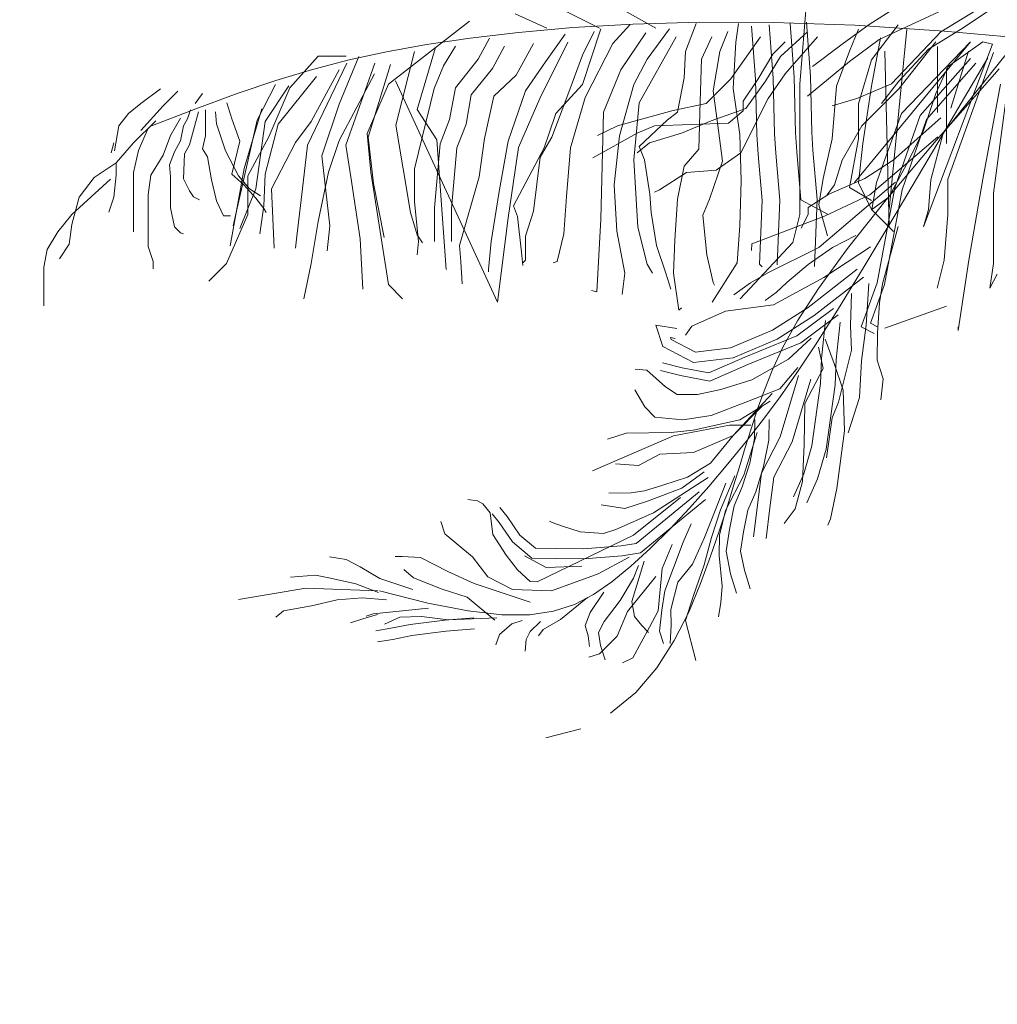
# Model space of a CAD drawing. Units: millimetres. Extents: x 595116 to 630915, y 909473 to 920225.
# Tile 67 of 134: x 629618.94 to 629629.07, y 919266.51 to 919276.71. Entities that reach past the tile are written whole.
import ezdxf

# ---------------------------------------------------------------- set-up
doc = ezdxf.new("R2010")
doc.units = ezdxf.units.MM
doc.layers.add('Dimension', color=3, linetype='Continuous', lineweight=18)
doc.layers.add('L-PLNT', color=85, linetype='Continuous', lineweight=13)
doc.styles.get("Standard").update_dxf_attribs({"font": 'arial.ttf'})
doc.dimstyles.new('ISO-25', dxfattribs={"dimtxt": 9, "dimasz": 6, "dimexe": 1.25, "dimexo": 0.625, "dimtad": 1, "dimlunit": 4, "dimtxsty": 'Standard', "dimcen": 2.5, "dimadec": 0, "dimazin": 0, "dimtfac": 1, "dimtmove": 0, "dimatfit": 3, "dimfxl": 1, "dimarcsym": 0})

# ---------------------------------------------------------------- blocks, each defined once
blk = doc.blocks.new('A$C4FB75ABC')
for p, q in [((2.1065, 2.3741), (2.087, 2.1315)), ((2.2781, 2.2963), (2.353, 2.344)), ((2.5983, 2.3508), (2.4757, 2.2759)), ((1.3881, 2.2867), (1.3008, 2.3255)), ((1.5337, 2.2867), (1.4367, 2.3352)), ((1.6891, 2.2867), (1.6017, 2.3352)), ((2.3054, 2.2555), (2.4825, 2.3372)), ((2.6119, 2.3372), (2.5302, 2.2827)), ((1.1746, 2.3061), (0.9513, 2.1315)), ((1.4598, 2.2878), (1.3106, 2.2744)), ((1.6258, 2.2976), (1.4598, 2.2878)), ((1.5376, 2.2844), (1.4866, 2.1313)), ((1.6179, 2.2954), (1.5705, 2.2443)), ((1.8099, 2.3026), (1.6258, 2.2976)), ((1.7274, 2.2844), (1.6654, 2.2006)), ((1.8004, 2.299), (1.7712, 2.2224)), ((2.0136, 2.3019), (1.8099, 2.3026)), ((1.9171, 2.299), (1.9098, 2.248)), ((1.9536, 2.2917), (1.9646, 2.1459)), ((2.0023, 2.2954), (2.0134, 2.1483)), ((2.2382, 2.2942), (2.0136, 2.3019)), ((2.0597, 2.2997), (2.0708, 2.1511)), ((2.1047, 2.3031), (2.1159, 2.1533)), ((2.2032, 2.2419), (2.2781, 2.2963)), ((2.2482, 2.2839), (2.2239, 2.2232)), ((2.4852, 2.2785), (2.2382, 2.2942)), ((2.3575, 2.296), (2.2846, 2.199)), ((2.3818, 2.2839), (2.3332, 1.7863)), ((1.1767, 2.2586), (1.0564, 2.241)), ((1.3106, 2.2744), (1.1767, 2.2586)), ((1.23, 2.2589), (1.1992, 2.2008)), ((1.4391, 2.2699), (1.3844, 2.1933)), ((1.5194, 2.2771), (1.4866, 2.2115)), ((1.6617, 2.2735), (1.5924, 2.1714)), ((1.7456, 2.2626), (1.6435, 2.0802)), ((1.8442, 2.2626), (1.815, 2.2006)), ((1.8879, 2.2771), (1.8661, 2.2224)), ((1.9783, 2.2623), (1.8966, 2.1465)), ((2.1078, 2.2759), (2.0328, 2.2078)), ((2.135, 2.2623), (2.0465, 2.1602)), ((2.3089, 2.2596), (2.2846, 2.1261)), ((2.4757, 2.2759), (2.3394, 2.1329)), ((2.5302, 2.2827), (2.4416, 2.2282)), ((2.6937, 2.2623), (2.4825, 1.9967)), ((2.7559, 2.2536), (2.4852, 2.2785)), ((1.0564, 2.241), (0.9464, 2.2213)), ((1.0815, 2.2334), (1.0304, 2.062)), ((1.1363, 2.237), (1.1034, 2.1823)), ((1.2713, 2.237), (1.2384, 2.175)), ((1.3515, 2.2443), (1.3041, 2.1568)), ((1.4464, 2.2479), (1.3687, 2.0927)), ((1.5705, 2.2443), (1.4939, 2.0948)), ((1.9098, 2.248), (1.9025, 2.1203)), ((2.0124, 2.2146), (2.0465, 2.2487)), ((2.1214, 2.1806), (2.2032, 2.2419)), ((2.2236, 2.1942), (2.3054, 2.2555)), ((2.5574, 2.2487), (2.2372, 1.8605)), ((2.462, 2.2487), (2.3599, 2.1193)), ((2.3667, 2.0512), (2.5574, 2.2487)), ((2.428, 1.738), (2.6187, 2.2419)), ((2.4668, 2.2354), (2.4668, 2.0533)), ((2.5915, 2.2487), (2.4961, 2.1806)), ((2.6187, 2.2419), (2.5915, 2.2487)), ((0.7572, 2.2091), (0.6795, 2.1218)), ((0.8348, 2.2091), (0.7572, 2.2091)), ((0.8699, 2.2079), (0.8151, 2.0766)), ((0.9464, 2.2213), (0.8429, 2.1986)), ((1.0231, 2.2224), (0.972, 2.0182)), ((1.4866, 2.2115), (1.4464, 2.1021)), ((1.7712, 2.2224), (1.7675, 2.1495)), ((1.8661, 2.2224), (1.8478, 2.113)), ((1.9715, 2.1465), (2.0124, 2.2146)), ((2.0328, 2.2078), (1.992, 2.1397)), ((2.2239, 2.2232), (2.1875, 2.1261)), ((2.3211, 2.2232), (2.3332, 1.7378)), ((2.4416, 2.2282), (2.3599, 2.1397)), ((2.5572, 2.203), (2.4187, 2.0449)), ((2.6056, 2.2048), (2.4676, 1.9701)), ((2.6209, 2.2188), (2.4948, 1.8695)), ((2.5518, 2.2232), (2.5032, 2.0655)), ((0.837, 2.1896), (0.7276, 1.9635)), ((0.8429, 2.1986), (0.7422, 2.1723)), ((0.9137, 2.1896), (0.8334, 1.9635)), ((0.9575, 2.186), (0.8954, 1.9854)), ((1.1034, 2.1823), (1.0779, 2.1203)), ((1.1992, 2.2008), (1.1362, 2.1221)), ((1.2384, 2.175), (1.18, 2.1021)), ((1.3844, 2.1933), (1.3297, 2.113)), ((1.6654, 2.2006), (1.6289, 2.1313)), ((1.815, 2.2006), (1.8113, 2.0838)), ((2.1078, 2.0989), (2.2236, 2.1942)), ((2.2846, 2.199), (2.2482, 2.0776)), ((2.5724, 2.1897), (2.4365, 2.0345)), ((2.4961, 2.1806), (2.462, 2.1057)), ((2.6368, 2.1742), (2.4628, 1.9766)), ((2.4911, 2.1747), (2.4911, 1.9684)), ((0.7422, 2.1723), (0.6405, 2.1416)), ((0.7531, 2.1531), (0.6473, 2.0218)), ((0.8151, 2.1714), (0.7385, 2.0291)), ((0.9125, 2.1606), (0.8154, 1.9763)), ((1.3041, 2.1568), (1.2421, 2.0984)), ((1.5924, 2.1714), (1.5449, 2.0547)), ((1.7675, 2.1495), (1.7493, 2.0547)), ((2.0465, 2.1602), (1.9988, 2.0921)), ((2.0134, 2.1483), (2.017, 1.9949)), ((2.0708, 2.1511), (2.0745, 1.9975)), ((2.1159, 2.1533), (2.1196, 1.9995)), ((0.6405, 2.1416), (0.5342, 2.1057)), ((0.64, 2.1313), (0.5889, 2.0328)), ((0.6765, 2.1276), (0.6108, 2.0291)), ((0.6795, 2.1218), (0.6213, 1.986)), ((0.9513, 2.1315), (0.8931, 1.9957)), ((1.2522, 1.53), (0.9707, 2.1412)), ((1.0779, 2.1203), (1.0231, 1.8978)), ((1.1362, 2.1221), (1.1203, 2.0346)), ((1.4866, 2.1313), (1.4136, 2.051)), ((1.6289, 2.1313), (1.5887, 1.989)), ((1.8966, 2.1465), (1.8285, 2.0784)), ((1.9025, 2.1203), (1.9208, 1.9927)), ((1.9306, 2.0852), (1.9715, 2.1465)), ((1.992, 2.1397), (1.9375, 2.0648)), ((1.9646, 2.1459), (1.9682, 1.9927)), ((2.087, 2.1315), (2.087, 1.7725)), ((2.1875, 2.1261), (2.1754, 1.9805)), ((2.3394, 2.1329), (2.244, 2.0921)), ((2.2846, 2.1261), (2.2604, 1.9684)), ((2.3599, 2.1397), (2.3122, 2.0784)), ((2.6404, 2.1315), (2.5918, 1.8695)), ((2.6598, 2.1218), (2.6209, 1.8307)), ((0.2683, 2.0784), (0.3228, 2.1193)), ((0.3296, 2.0716), (0.3705, 2.1125)), ((0.4182, 2.0784), (0.4386, 2.1057)), ((0.5342, 2.1057), (0.4195, 2.0639)), ((1.18, 2.1021), (1.1654, 2.0218)), ((1.2421, 2.0984), (1.2165, 1.9817)), ((1.3297, 2.113), (1.2822, 1.9744)), ((1.3687, 2.0927), (1.3105, 1.9569)), ((1.4464, 2.1021), (1.4026, 1.9854)), ((1.4939, 2.0948), (1.4537, 1.9562)), ((1.8478, 2.113), (1.8624, 2.0036)), ((2.3599, 2.1193), (2.2577, 2.0172)), ((2.462, 2.1057), (2.428, 2.0035)), ((0.2342, 2.0512), (0.2683, 2.0784)), ((0.2683, 2.0035), (0.3296, 2.0716)), ((0.505, 2.0802), (0.5196, 2.0364)), ((0.8151, 2.0766), (0.7677, 1.9343)), ((1.6435, 2.0802), (1.6289, 1.9234)), ((1.8285, 2.0784), (1.7331, 2.058)), ((1.8113, 2.0838), (1.8077, 1.9526)), ((1.9988, 2.0921), (1.9238, 1.9422)), ((1.9306, 2.058), (1.9306, 2.0852)), ((2.244, 2.0921), (2.1759, 2.0716)), ((2.2482, 2.0776), (2.2482, 1.9805)), ((0.207, 2.0172), (0.2342, 2.0512)), ((0.4195, 2.0639), (0.2927, 2.0154)), ((0.4049, 2.0609), (0.3966, 2.0361)), ((0.427, 2.0554), (0.4021, 1.9643)), ((0.4463, 2.0609), (0.4463, 1.9892)), ((0.4739, 2.0554), (0.4767, 2.0223)), ((0.6018, 2.0636), (0.5533, 1.8986)), ((1.0304, 2.062), (1.0852, 1.9781)), ((1.4136, 2.051), (1.3953, 1.9963)), ((1.5449, 2.0547), (1.5376, 1.7593)), ((1.7331, 2.058), (1.5832, 2.0172)), ((1.7493, 2.0547), (1.7201, 2.0328)), ((1.9375, 2.0648), (1.8421, 2.0308)), ((1.8898, 2.024), (1.9306, 2.058)), ((2.2985, 1.8605), (2.3667, 2.0512)), ((2.4756, 2.0387), (2.3438, 1.9217)), ((2.4187, 2.0449), (2.3489, 1.8456)), ((0.195, 1.9478), (0.207, 2.0172)), ((0.3092, 2.0308), (0.2479, 1.9695)), ((0.3773, 2.0376), (0.3501, 1.9899)), ((0.3855, 2.0168), (0.3773, 1.9754)), ((0.3966, 2.0361), (0.3855, 2.0168)), ((0.4767, 2.0223), (0.5015, 1.9478)), ((0.5196, 2.0364), (0.5415, 1.9744)), ((0.5889, 2.0328), (0.5232, 1.741)), ((0.6108, 2.0291), (0.5853, 1.8431)), ((0.6473, 2.0218), (0.6108, 1.8833)), ((0.7385, 2.0291), (0.6947, 1.9708)), ((0.972, 2.0182), (1.0122, 1.7775)), ((1.1203, 2.0346), (1.0939, 1.9669)), ((1.1654, 2.0218), (1.1399, 1.9562)), ((1.5832, 2.0172), (1.5287, 1.9899)), ((1.6377, 1.9967), (1.6854, 2.0172)), ((1.7201, 2.0328), (1.6435, 1.9598)), ((1.6854, 2.0172), (1.8898, 2.024)), ((1.8421, 2.0308), (1.7603, 1.9967)), ((2.2577, 2.0172), (2.2032, 1.9218)), ((2.4365, 2.0345), (2.3686, 1.8404)), ((0.2887, 2.0103), (0.2615, 1.9491)), ((0.3501, 1.9899), (0.3296, 1.9354)), ((0.4463, 1.9892), (0.438, 1.9533)), ((0.6213, 1.986), (0.563, 1.8792)), ((0.8931, 1.9957), (0.9028, 1.8889)), ((0.8954, 1.9854), (0.91, 1.8577)), ((1.4026, 1.9854), (1.3698, 1.9307)), ((1.3953, 1.9963), (1.3807, 1.9562)), ((1.5151, 1.9286), (1.6377, 1.9967)), ((1.5887, 1.989), (1.5741, 1.8541)), ((1.7603, 1.9967), (1.6718, 1.9695)), ((1.8624, 2.0036), (1.8734, 1.9197)), ((1.9208, 1.9927), (1.9244, 1.865)), ((1.9682, 1.9927), (1.9719, 1.938)), ((2.017, 1.9949), (2.0206, 1.9417)), ((2.0745, 1.9975), (2.0779, 1.946)), ((2.1196, 1.9995), (2.1229, 1.9495)), ((2.4673, 1.986), (2.2802, 1.8264)), ((2.428, 2.0035), (2.3871, 1.9218)), ((2.4825, 1.9967), (2.4484, 1.8673)), ((0.1865, 1.9422), (0.1934, 1.9695)), ((0.2479, 1.9695), (0.2002, 1.915)), ((0.3773, 1.9754), (0.3607, 1.945)), ((0.4021, 1.9643), (0.3883, 1.9395)), ((0.5415, 1.9744), (0.5196, 1.8833)), ((0.6947, 1.9708), (0.629, 1.8431)), ((0.7276, 1.9635), (0.713, 1.8358)), ((0.8154, 1.9763), (0.7863, 1.8889)), ((0.8334, 1.9635), (0.848, 1.876)), ((1.0939, 1.9669), (1.0786, 1.7905)), ((1.0852, 1.9781), (1.1107, 1.6207)), ((1.2165, 1.9817), (1.2019, 1.876)), ((1.2822, 1.9744), (1.2567, 1.8358)), ((1.3105, 1.9569), (1.2814, 1.7628)), ((1.6718, 1.9695), (1.6377, 1.9422)), ((1.6435, 1.9598), (1.6581, 1.9234)), ((2.1754, 1.9805), (2.1511, 1.8713)), ((2.2482, 1.9805), (2.2239, 1.847)), ((2.2604, 1.9684), (2.2482, 1.8591)), ((2.4628, 1.9766), (2.3249, 1.8127)), ((2.4676, 1.9701), (2.3552, 1.7802)), ((0.2615, 1.9491), (0.2479, 1.8878)), ((0.3296, 1.9354), (0.2956, 1.881)), ((0.3607, 1.945), (0.3469, 1.9091)), ((0.3883, 1.9395), (0.3855, 1.8705)), ((0.438, 1.9533), (0.4518, 1.9312)), ((0.4518, 1.9312), (0.4629, 1.8677)), ((0.5015, 1.9478), (0.5374, 1.8788)), ((0.7677, 1.9343), (0.7896, 1.741)), ((1.1399, 1.9562), (1.1253, 1.7884)), ((1.3807, 1.9562), (1.2968, 1.7957)), ((1.3698, 1.9307), (1.3515, 1.7811)), ((1.4537, 1.9562), (1.4428, 1.8213)), ((1.8077, 1.9526), (1.7675, 1.9051)), ((1.9238, 1.9422), (1.8557, 1.8946)), ((1.9719, 1.938), (1.9828, 1.8103)), ((2.0206, 1.9417), (2.0317, 1.8114)), ((2.0779, 1.946), (2.0893, 1.8127)), ((2.1229, 1.9495), (2.1345, 1.8136)), ((0.2002, 1.915), (0.1389, 1.8742)), ((0.2002, 1.915), (0.2002, 1.881)), ((0.3469, 1.9091), (0.3497, 1.876)), ((1.6289, 1.9234), (1.6398, 1.7374)), ((1.6581, 1.9234), (1.6727, 1.8285)), ((1.7675, 1.9051), (1.7493, 1.814)), ((1.8734, 1.9197), (1.8369, 1.814)), ((2.2032, 1.9218), (2.1827, 1.8537)), ((2.3438, 1.9217), (2.2657, 1.8718)), ((2.3871, 1.9218), (2.3326, 1.8197)), ((0.2002, 1.881), (0.1934, 1.8197)), ((0.2479, 1.8878), (0.2479, 1.8061)), ((0.2956, 1.881), (0.2887, 1.8265)), ((0.3497, 1.876), (0.3497, 1.8512)), ((0.5196, 1.8833), (0.5524, 1.8541)), ((0.5533, 1.8986), (0.5339, 1.7919)), ((0.5374, 1.8788), (0.5678, 1.8429)), ((0.563, 1.8792), (0.563, 1.7725)), ((0.6108, 1.8833), (0.6072, 1.7957)), ((0.7863, 1.8889), (0.7572, 1.7531)), ((0.848, 1.876), (0.8735, 1.7045)), ((0.9028, 1.8889), (0.9513, 1.5785)), ((1.0231, 1.8978), (1.0231, 1.8067)), ((1.2019, 1.876), (1.1472, 1.6863)), ((1.7739, 1.8878), (1.699, 1.8401)), ((1.8557, 1.8946), (1.7739, 1.8878)), ((0.1844, 1.8695), (0.0777, 1.7725)), ((0.1389, 1.8742), (0.098, 1.8197)), ((0.3497, 1.8512), (0.3497, 1.7904)), ((0.3855, 1.8705), (0.4021, 1.8374)), ((0.4629, 1.8677), (0.4767, 1.8098)), ((0.5524, 1.8541), (0.5853, 1.8176)), ((0.91, 1.8577), (0.9392, 1.7082)), ((1.5741, 1.8541), (1.5814, 1.7264)), ((1.9244, 1.865), (1.9208, 1.741)), ((2.3505, 1.8613), (2.1386, 1.6813)), ((2.1511, 1.8713), (2.1389, 1.7985)), ((2.1827, 1.8537), (2.1623, 1.8265)), ((2.2657, 1.8718), (2.167, 1.8279)), ((2.2482, 1.8591), (2.2846, 1.7863)), ((2.2849, 1.7856), (2.2985, 1.8605)), ((2.4484, 1.8673), (2.4416, 1.7856)), ((2.4948, 1.8695), (2.4948, 1.7725)), ((2.5918, 1.8695), (2.553, 1.6464)), ((0.2887, 1.8265), (0.2887, 1.7516)), ((0.4021, 1.8374), (0.4132, 1.8208)), ((0.5853, 1.8431), (0.5415, 1.7337)), ((0.5678, 1.8429), (0.5982, 1.8236)), ((0.629, 1.8431), (0.6363, 1.679)), ((0.713, 1.8358), (0.6984, 1.7118)), ((1.2567, 1.8358), (1.2348, 1.6973)), ((1.4428, 1.8213), (1.4355, 1.7191)), ((1.6727, 1.8285), (1.6763, 1.7775)), ((1.699, 1.8401), (1.6854, 1.8333)), ((2.167, 1.8279), (2.1099, 1.791)), ((2.2802, 1.8264), (2.1549, 1.7678)), ((2.2239, 1.847), (2.2846, 1.8106)), ((2.3489, 1.8456), (2.3004, 1.5838)), ((2.3686, 1.8404), (2.32, 1.5785)), ((2.6209, 1.8307), (2.6209, 1.6367)), ((0.098, 1.8197), (0.0775, 1.7448)), ((0.1934, 1.8197), (0.1797, 1.7788)), ((0.2479, 1.8061), (0.2479, 1.7448)), ((0.4132, 1.8208), (0.4297, 1.8125)), ((0.4767, 1.8098), (0.496, 1.7684)), ((0.5853, 1.8176), (0.6072, 1.7884)), ((0.6072, 1.7957), (0.5962, 1.7191)), ((1.0231, 1.8067), (1.0341, 1.6973)), ((1.2968, 1.7957), (1.3078, 1.7665)), ((1.7493, 1.814), (1.742, 1.7009)), ((1.8369, 1.814), (1.8186, 1.7702)), ((1.9828, 1.8103), (1.9755, 1.6352)), ((2.0317, 1.8114), (2.0243, 1.6332)), ((2.0893, 1.8127), (2.1647, 1.7725)), ((2.1345, 1.8136), (2.1268, 1.6289)), ((2.1389, 1.7985), (2.1632, 1.7135)), ((2.3249, 1.8127), (2.2184, 1.678)), ((2.3326, 1.8197), (2.2849, 1.7856)), ((0.0777, 1.7725), (0.0388, 1.724)), ((0.3497, 1.7904), (0.3607, 1.738)), ((0.496, 1.7684), (0.5153, 1.7684)), ((0.563, 1.7725), (0.5048, 1.6367)), ((0.5339, 1.7919), (0.5145, 1.6852)), ((0.6072, 1.7884), (0.6144, 1.7775)), ((1.0122, 1.7775), (1.0304, 1.7155)), ((1.0786, 1.7905), (1.0786, 1.6973)), ((1.1253, 1.7884), (1.1253, 1.7665)), ((1.1253, 1.7665), (1.1253, 1.7301)), ((1.3078, 1.7665), (1.3187, 1.6681)), ((1.3515, 1.7811), (1.3297, 1.7118)), ((1.6763, 1.7775), (1.6909, 1.6863)), ((1.8186, 1.7702), (1.8296, 1.6608)), ((2.1549, 1.7678), (1.9538, 1.6913)), ((2.087, 1.7725), (2.0676, 1.6949)), ((2.1096, 1.7722), (2.0903, 1.7347)), ((2.1099, 1.791), (2.1096, 1.7722)), ((2.3552, 1.7802), (2.2641, 1.6283)), ((2.2846, 1.7863), (2.3453, 1.7256)), ((2.4416, 1.7856), (2.428, 1.738)), ((2.4948, 1.7725), (2.485, 1.6464)), ((0.0775, 1.7448), (0.0707, 1.6903)), ((0.2479, 1.7448), (0.2479, 1.7243)), ((0.2887, 1.7516), (0.2887, 1.6835)), ((0.7572, 1.7531), (0.7377, 1.6367)), ((0.7896, 1.741), (0.7823, 1.6717)), ((1.2814, 1.7628), (1.2522, 1.53)), ((1.5376, 1.7593), (1.5267, 1.5587)), ((1.9208, 1.741), (1.9135, 1.6389)), ((0.0388, 1.724), (0.0097, 1.6755)), ((0.3607, 1.738), (0.3773, 1.7214)), ((0.3773, 1.7214), (0.3855, 1.7187)), ((1.0304, 1.7155), (1.045, 1.6936)), ((1.1253, 1.7301), (1.1253, 1.6973)), ((1.4355, 1.7191), (1.4172, 1.6425)), ((1.5814, 1.7264), (1.6033, 1.6097)), ((1.6398, 1.7374), (1.6654, 1.6352)), ((2.2409, 1.7138), (2.1763, 1.6807)), ((2.3582, 1.7386), (2.3145, 1.5808)), ((0.0707, 1.6903), (0.0435, 1.6494)), ((0.6984, 1.7118), (0.6947, 1.679)), ((0.8735, 1.7045), (0.8808, 1.566)), ((1.0341, 1.6973), (1.0304, 1.6608)), ((1.1472, 1.6863), (1.1509, 1.6425)), ((1.2348, 1.6973), (1.2275, 1.6207)), ((1.3297, 1.7118), (1.3297, 1.6462)), ((1.6909, 1.6863), (1.7164, 1.6097)), ((1.742, 1.7009), (1.7383, 1.6097)), ((2.0676, 1.6949), (1.922, 1.5397)), ((1.9538, 1.6913), (1.9536, 1.6725)), ((0.0097, 1.6755), (0, 1.627)), ((0.2887, 1.6835), (0.3024, 1.6426)), ((1.3187, 1.6681), (1.3224, 1.6316)), ((1.8296, 1.6608), (1.8478, 1.5842)), ((2.1386, 1.6813), (1.998, 1.6115)), ((2.1763, 1.6807), (2.1096, 1.6345)), ((2.2184, 1.678), (2.1385, 1.568)), ((2.2819, 1.6831), (2.1525, 1.5981)), ((0.3024, 1.6426), (0.3024, 1.6222)), ((0.5048, 1.6367), (0.4562, 1.5882)), ((0.7377, 1.6367), (0.7183, 1.5397)), ((1.1509, 1.6425), (1.1545, 1.5805)), ((1.3297, 1.6462), (1.3224, 1.6389)), ((1.4172, 1.6425), (1.4063, 1.6389)), ((1.6654, 1.6352), (1.68, 1.6097)), ((1.9135, 1.6389), (1.8444, 1.53)), ((1.9755, 1.6352), (1.9828, 1.628)), ((2.1096, 1.6345), (2.0504, 1.5844)), ((2.485, 1.6464), (2.4656, 1.5688)), ((2.553, 1.6464), (2.5239, 1.4523)), ((2.6209, 1.6367), (2.6112, 1.5688)), ((0, 1.627), (0, 1.5494)), ((1.2275, 1.6207), (1.2275, 1.6134)), ((1.6033, 1.6097), (1.596, 1.5514)), ((1.7164, 1.6097), (1.731, 1.566)), ((1.7383, 1.6097), (1.7529, 1.5076)), ((1.998, 1.6115), (1.9504, 1.5839)), ((2.2452, 1.6213), (2.1098, 1.5157)), ((2.2641, 1.6283), (2.1904, 1.5079)), ((2.6112, 1.5688), (2.6307, 1.6076)), ((0.9513, 1.5785), (0.9901, 1.5397)), ((1.8478, 1.5842), (1.8515, 1.5769)), ((1.9504, 1.5839), (1.9047, 1.5506)), ((2.1525, 1.5981), (2.0137, 1.5227)), ((2.0504, 1.5844), (2.0217, 1.5565)), ((2.2623, 1.5995), (2.1258, 1.493)), ((2.3004, 1.5838), (2.256, 1.4617)), ((2.2767, 1.5813), (2.2695, 1.4664)), ((2.32, 1.5785), (2.2812, 1.4717)), ((2.3145, 1.5808), (2.3062, 1.5281)), ((0, 1.5494), (0, 1.5203)), ((1.5267, 1.5587), (1.5121, 1.5623)), ((2.0217, 1.5565), (1.9912, 1.5343)), ((2.1385, 1.568), (2.0803, 1.4783)), ((2.2292, 1.5537), (2.2261, 1.4651)), ((2.0137, 1.5227), (1.8814, 1.5056)), ((2.3062, 1.5281), (2.3013, 1.4452)), ((1.7529, 1.5076), (1.7602, 1.5149)), ((1.8814, 1.5056), (1.7884, 1.4636)), ((2.1098, 1.5157), (2.0109, 1.453)), ((2.1796, 1.5129), (2.0785, 1.437)), ((2.1927, 1.4954), (2.0894, 1.4177)), ((2.1904, 1.5079), (2.1298, 1.4122)), ((2.4911, 1.5193), (2.3211, 1.4586)), ((2.1258, 1.493), (2.0238, 1.4284)), ((2.0803, 1.4783), (2.039, 1.4043)), ((2.1578, 1.4791), (2.1468, 1.3743)), ((2.1979, 1.4749), (2.187, 1.3714)), ((2.2812, 1.4717), (2.3006, 1.462)), ((1.7084, 1.4073), (1.6895, 1.4666)), ((1.6895, 1.4666), (1.747, 1.4576)), ((1.7884, 1.4636), (1.7711, 1.4393)), ((2.0109, 1.453), (1.8951, 1.4036)), ((2.2261, 1.4651), (2.2289, 1.3972)), ((2.256, 1.4617), (2.2916, 1.4439)), ((2.2695, 1.4664), (2.2568, 1.3685)), ((2.3013, 1.4452), (2.3002, 1.3698)), ((2.5239, 1.4523), (2.5239, 1.462)), ((1.7313, 1.4266), (1.7295, 1.4323)), ((1.7295, 1.4323), (1.7427, 1.4302)), ((1.7987, 1.3918), (1.7313, 1.4266)), ((2.0238, 1.4284), (1.9024, 1.3766)), ((2.0785, 1.437), (1.9344, 1.3786)), ((2.0894, 1.4177), (1.9429, 1.3584)), ((2.1181, 1.4308), (2.055, 1.3732)), ((2.1569, 1.4277), (2.1816, 1.3609)), ((1.7936, 1.3632), (1.7084, 1.4073)), ((1.8951, 1.4036), (1.7987, 1.3918)), ((2.039, 1.4043), (2.0098, 1.3416)), ((2.1298, 1.4122), (2.0784, 1.3347)), ((2.1385, 1.406), (2.1509, 1.3473)), ((2.2289, 1.3972), (2.1929, 1.2544)), ((1.7623, 1.3489), (1.7078, 1.3628)), ((1.9024, 1.3766), (1.7936, 1.3632)), ((1.9344, 1.3786), (1.8357, 1.3347)), ((2.055, 1.3732), (1.9542, 1.3161)), ((2.1468, 1.3743), (2.1439, 1.3053)), ((2.1816, 1.3609), (2.2062, 1.287)), ((2.187, 1.3714), (2.1842, 1.3016)), ((2.2568, 1.3685), (2.2516, 1.2668)), ((2.3002, 1.3698), (2.3165, 1.3187)), ((1.6641, 1.3427), (1.6321, 1.345)), ((1.7163, 1.2967), (1.6641, 1.3427)), ((1.7575, 1.3275), (1.7024, 1.3416)), ((1.8357, 1.3347), (1.7623, 1.3489)), ((1.9429, 1.3584), (1.8383, 1.3119)), ((2.0098, 1.3416), (1.9878, 1.2857)), ((2.0811, 1.3502), (2.0312, 1.2905)), ((2.0784, 1.3347), (2.0319, 1.2687)), ((2.1509, 1.3473), (2.1005, 1.25)), ((1.8383, 1.3119), (1.7575, 1.3275)), ((1.9542, 1.3161), (1.869, 1.289)), ((2.0829, 1.3276), (2.0324, 1.158)), ((2.1165, 1.3176), (2.065, 1.1449)), ((2.1439, 1.3053), (2.1195, 1.1332)), ((2.3165, 1.3187), (2.31, 1.2603)), ((1.6589, 1.2409), (1.6313, 1.2885)), ((1.7481, 1.2755), (1.7163, 1.2967)), ((1.869, 1.289), (1.8046, 1.2748)), ((2.0103, 1.2776), (1.903, 1.1622)), ((2.0312, 1.2905), (1.9421, 1.2559)), ((1.9878, 1.2857), (1.9691, 1.2327)), ((2.1842, 1.3016), (2.1591, 1.1247)), ((2.2062, 1.287), (2.2097, 1.1745)), ((1.8046, 1.2748), (1.7481, 1.2755)), ((1.9421, 1.2559), (1.8416, 1.2177)), ((2.0043, 1.257), (1.9206, 1.2053)), ((2.0319, 1.2687), (1.9864, 1.2075)), ((2.1929, 1.2544), (2.1754, 1.2112)), ((2.2516, 1.2668), (2.22, 1.1691)), ((1.6868, 1.2123), (1.6589, 1.2409)), ((1.9834, 1.244), (1.903, 1.1622)), ((1.9691, 1.2327), (1.952, 1.1808)), ((2.1005, 1.25), (2.0989, 1.1369)), ((1.7641, 1.2056), (1.6868, 1.2123)), ((1.8416, 1.2177), (1.7641, 1.2056)), ((1.9206, 1.2053), (1.792, 1.1769)), ((1.9864, 1.2075), (1.9386, 1.1458)), ((1.9621, 1.2066), (1.9614, 1.1536)), ((2.0017, 1.2061), (2.001, 1.1495)), ((2.1754, 1.2112), (2.1606, 1.1002)), ((1.7315, 1.1702), (1.607, 1.1681)), ((1.792, 1.1769), (1.7315, 1.1702)), ((1.7376, 1.1613), (1.8929, 1.1904)), ((1.8929, 1.1904), (1.9511, 1.1904)), ((1.9692, 1.1707), (1.9317, 1.0524)), ((1.952, 1.1808), (1.9358, 1.129)), ((2.2097, 1.1745), (2.1886, 1.0162)), ((1.5143, 1.0642), (1.7376, 1.1613)), ((1.607, 1.1681), (1.5558, 1.1518)), ((1.903, 1.1622), (1.793, 1.1147)), ((1.903, 1.1622), (1.8397, 1.0857)), ((1.9386, 1.1458), (1.8882, 1.0835)), ((1.9614, 1.1536), (1.9482, 1.0859)), ((2.0324, 1.158), (1.9806, 1.0581)), ((2.001, 1.1495), (1.9867, 1.0762)), ((2.065, 1.1449), (2.0146, 1.0475)), ((1.793, 1.1147), (1.7005, 1.1103)), ((1.9358, 1.129), (1.9198, 1.076)), ((2.0989, 1.1369), (2.0937, 1.0351)), ((2.1195, 1.1332), (2.0972, 1.056)), ((2.1591, 1.1247), (2.1353, 1.0421)), ((1.7005, 1.1103), (1.6416, 1.079)), ((1.6416, 1.079), (1.5775, 1.0837)), ((1.8224, 1.0615), (1.7614, 1.017)), ((1.8397, 1.0857), (1.7769, 1.047)), ((1.8882, 1.0835), (1.8359, 1.0215)), ((1.9198, 1.076), (1.903, 1.0206)), ((1.9482, 1.0859), (1.9278, 1.0204)), ((1.9867, 1.0762), (1.965, 1.0067)), ((1.8335, 1.0462), (1.6831, 0.9483)), ((1.7769, 1.047), (1.7087, 1.0253)), ((1.9071, 1.0509), (1.8681, 0.9571)), ((1.9317, 1.0524), (1.8813, 0.9551)), ((1.9806, 1.0581), (1.9586, 0.8825)), ((2.0146, 1.0475), (2.004, 0.9628)), ((2.0972, 1.056), (2.0692, 0.9929)), ((2.0937, 1.0351), (2.0738, 0.96)), ((2.1353, 1.0421), (2.1061, 0.9765)), ((1.6576, 1.009), (1.6216, 1.0039)), ((1.8084, 1.007), (1.6348, 0.8642)), ((1.7087, 1.0253), (1.6576, 1.009)), ((1.7614, 1.017), (1.6666, 0.9806)), ((1.8359, 1.0215), (1.7823, 0.9612)), ((1.8823, 1.0305), (1.8549, 0.9592)), ((1.903, 1.0206), (1.8847, 0.9618)), ((1.9278, 1.0204), (1.9055, 0.9679)), ((1.965, 1.0067), (1.9435, 0.9561)), ((2.1886, 1.0162), (2.171, 0.9318)), ((1.1969, 0.9814), (1.1705, 0.9855)), ((1.2119, 0.9737), (1.1969, 0.9814)), ((1.6216, 1.0039), (1.5594, 1.0028)), ((1.6666, 0.9806), (1.6041, 0.9607)), ((1.7573, 0.9907), (1.6276, 0.8869)), ((1.8259, 0.9857), (1.6466, 0.8382)), ((1.2323, 0.9489), (1.2119, 0.9737)), ((1.2793, 0.9388), (1.2589, 0.9636)), ((1.6041, 0.9607), (1.5382, 0.9711)), ((1.7823, 0.9612), (1.7281, 0.9036)), ((1.8549, 0.9592), (1.8236, 0.8804)), ((1.8681, 0.9571), (1.8425, 0.8802)), ((1.8847, 0.9618), (1.8642, 0.8983)), ((1.8813, 0.9551), (1.8652, 0.8874)), ((1.9055, 0.9679), (1.8924, 0.9029)), ((1.9435, 0.9561), (1.9314, 0.8959)), ((2.004, 0.9628), (1.9934, 0.8781)), ((2.0738, 0.96), (2.043, 0.9189)), ((1.107, 0.8902), (1.0961, 0.9243)), ((1.239, 0.8884), (1.2323, 0.9489)), ((1.2572, 0.9222), (1.2376, 0.9461)), ((1.3144, 0.8874), (1.2793, 0.9388)), ((1.4036, 0.922), (1.3961, 0.9259)), ((1.6831, 0.9483), (1.5787, 0.9026)), ((2.171, 0.9318), (2.164, 0.9142)), ((1.2938, 0.8688), (1.2572, 0.9222)), ((1.4317, 0.9122), (1.4036, 0.922)), ((1.4805, 0.8964), (1.4317, 0.9122)), ((1.5787, 0.9026), (1.5446, 0.8918)), ((1.7281, 0.9036), (1.6739, 0.8498)), ((1.7864, 0.9186), (1.765, 0.868)), ((1.8642, 0.8983), (1.8405, 0.829)), ((1.8924, 0.9029), (1.8829, 0.8424)), ((1.1405, 0.8634), (1.107, 0.8902)), ((1.2759, 0.8314), (1.239, 0.8884)), ((1.3573, 0.851), (1.3144, 0.8874)), ((1.6276, 0.8869), (1.3617, 0.7585)), ((1.5446, 0.8918), (1.4805, 0.8964)), ((1.8236, 0.8804), (1.7906, 0.8073)), ((1.8425, 0.8802), (1.8226, 0.805)), ((1.8652, 0.8874), (1.8644, 0.8308)), ((1.9314, 0.8959), (1.9231, 0.8432)), ((1.1834, 0.827), (1.1405, 0.8634)), ((1.347, 0.8236), (1.2938, 0.8688)), ((1.4139, 0.8502), (1.3573, 0.851)), ((1.4893, 0.8492), (1.4139, 0.8502)), ((1.5932, 0.8572), (1.4893, 0.8492)), ((1.6348, 0.8642), (1.5932, 0.8572)), ((1.6739, 0.8498), (1.6204, 0.8011)), ((1.7347, 0.8614), (1.7065, 0.7946)), ((1.765, 0.868), (1.7376, 0.7967)), ((1.9231, 0.8432), (1.9337, 0.7903)), ((0.8346, 0.8198), (0.7888, 0.827)), ((0.8736, 0.7996), (0.8346, 0.8198)), ((0.9891, 0.8277), (0.9703, 0.828)), ((1.04, 0.8252), (0.9891, 0.8277)), ((1.1149, 0.7864), (1.04, 0.8252)), ((1.226, 0.7717), (1.1834, 0.827)), ((1.3074, 0.7913), (1.2759, 0.8314)), ((1.3863, 0.7981), (1.3265, 0.8298)), ((1.4135, 0.8227), (1.347, 0.8236)), ((1.4902, 0.8216), (1.4135, 0.8227)), ((1.5965, 0.8298), (1.4902, 0.8216)), ((1.6154, 0.8267), (1.5299, 0.7807)), ((1.6466, 0.8382), (1.5965, 0.8298)), ((1.8405, 0.829), (1.8129, 0.7535)), ((1.8644, 0.8308), (1.8727, 0.7459)), ((1.8829, 0.8424), (1.8952, 0.7804)), ((0.9273, 0.7678), (0.8736, 0.7996)), ((1.0204, 0.7689), (0.9943, 0.7918)), ((1.3428, 0.7588), (1.3074, 0.7913)), ((1.4848, 0.8016), (1.3863, 0.7981)), ((1.6204, 0.8011), (1.5682, 0.7585)), ((1.6567, 0.8148), (1.6231, 0.704)), ((1.6415, 0.8037), (1.6278, 0.7681)), ((1.7065, 0.7946), (1.696, 0.6785)), ((1.7376, 0.7967), (1.7141, 0.733)), ((1.7906, 0.8073), (1.7502, 0.757)), ((1.8226, 0.805), (1.7931, 0.7206)), ((1.9337, 0.7903), (1.9499, 0.7392)), ((0.7503, 0.7767), (0.6814, 0.7711)), ((0.7912, 0.768), (0.7503, 0.7767)), ((0.8615, 0.7523), (0.7912, 0.768)), ((1.0187, 0.737), (0.9273, 0.7678)), ((1.0992, 0.7376), (1.0204, 0.7689)), ((1.188, 0.7534), (1.1149, 0.7864)), ((1.2935, 0.7368), (1.226, 0.7717)), ((1.5299, 0.7807), (1.4009, 0.7335)), ((1.6278, 0.7681), (1.5911, 0.7064)), ((1.6891, 0.7732), (1.6114, 0.6762)), ((1.8952, 0.7804), (1.9122, 0.7271)), ((0.7236, 0.7411), (0.5379, 0.7092)), ((0.9219, 0.7334), (0.7236, 0.7411)), ((0.9235, 0.7285), (0.8615, 0.7523)), ((1.1687, 0.7159), (1.0992, 0.7376)), ((1.342, 0.7022), (1.188, 0.7534)), ((1.4009, 0.7335), (1.2935, 0.7368)), ((1.3617, 0.7585), (1.3428, 0.7588)), ((1.5682, 0.7585), (1.5172, 0.7231)), ((1.7502, 0.757), (1.7303, 0.6818)), ((1.8129, 0.7535), (1.7799, 0.6746)), ((1.8727, 0.7459), (1.8683, 0.7007)), ((0.8101, 0.7087), (0.7393, 0.6917)), ((0.879, 0.7143), (0.8101, 0.7087)), ((0.9462, 0.7085), (0.879, 0.7143)), ((1.0599, 0.6997), (0.9265, 0.7333)), ((1.2451, 0.6526), (1.1687, 0.7159)), ((1.5006, 0.7151), (1.4262, 0.6539)), ((1.5172, 0.7231), (1.4647, 0.6957)), ((1.5461, 0.7296), (1.5076, 0.6736)), ((1.7141, 0.733), (1.7058, 0.6803)), ((1.7931, 0.7206), (1.7714, 0.6511)), ((0.7393, 0.6917), (0.6621, 0.678)), ((1.0623, 0.6856), (0.9095, 0.6697)), ((1.1712, 0.6779), (1.0599, 0.6997)), ((1.4647, 0.6957), (1.4072, 0.6768)), ((1.5911, 0.7064), (1.5469, 0.6485)), ((1.6231, 0.704), (1.6301, 0.6625)), ((1.7058, 0.6803), (1.6993, 0.6219)), ((1.7303, 0.6818), (1.7316, 0.6384)), ((1.8683, 0.7007), (1.8621, 0.6612)), ((0.6621, 0.678), (0.6405, 0.6602)), ((0.8811, 0.6557), (0.847, 0.6449)), ((0.9209, 0.6684), (0.8811, 0.6557)), ((0.9095, 0.6697), (0.8898, 0.6634)), ((0.9832, 0.6605), (0.9403, 0.6414)), ((1.0423, 0.6629), (0.9832, 0.6605)), ((1.1074, 0.6526), (1.011, 0.6408)), ((1.1159, 0.6537), (1.0423, 0.6629)), ((1.1867, 0.6591), (1.1074, 0.6526)), ((1.2504, 0.6584), (1.1159, 0.6537)), ((1.2639, 0.6673), (1.1712, 0.6779)), ((1.3414, 0.6671), (1.2639, 0.6673)), ((1.4072, 0.6768), (1.3414, 0.6671)), ((1.4262, 0.6539), (1.3787, 0.6263)), ((1.5076, 0.6736), (1.4939, 0.6379)), ((1.6114, 0.6762), (1.5823, 0.6082)), ((1.6301, 0.6625), (1.6505, 0.6377)), ((1.696, 0.6785), (1.6713, 0.6328)), ((1.7799, 0.6746), (1.74, 0.5958)), ((0.9581, 0.6302), (0.9165, 0.6232)), ((1.011, 0.6408), (0.9581, 0.6302)), ((1.1893, 0.628), (1.1106, 0.6216)), ((1.2921, 0.6426), (1.2578, 0.6129)), ((1.3206, 0.6516), (1.2921, 0.6426)), ((1.3714, 0.649), (1.3428, 0.6211)), ((1.3787, 0.6263), (1.3652, 0.6095)), ((1.4939, 0.6379), (1.5029, 0.6095)), ((1.5469, 0.6485), (1.5314, 0.6186)), ((1.6713, 0.6328), (1.6256, 0.5484)), ((1.6505, 0.6377), (1.6691, 0.6186)), ((1.7316, 0.6384), (1.729, 0.5876)), ((1.7714, 0.6511), (1.8, 0.5413)), ((0.9632, 0.5994), (0.9216, 0.5925)), ((1.016, 0.61), (0.9632, 0.5994)), ((1.1106, 0.6216), (1.016, 0.61)), ((1.2578, 0.6129), (1.2479, 0.5847)), ((1.3311, 0.5987), (1.3288, 0.5666)), ((1.3428, 0.6211), (1.3311, 0.5987)), ((1.5029, 0.6095), (1.5063, 0.5793)), ((1.5314, 0.6186), (1.5365, 0.5827)), ((1.5823, 0.6082), (1.5337, 0.5597)), ((1.6993, 0.6219), (1.7101, 0.5878)), ((1.5365, 0.5827), (1.5492, 0.5429)), ((1.74, 0.5958), (1.6917, 0.5207)), ((1.5337, 0.5597), (1.5046, 0.55)), ((1.6256, 0.5484), (1.5974, 0.5343)), ((1.6917, 0.5207), (1.6336, 0.4527)), ((1.6336, 0.4527), (1.5642, 0.3956)), ((1.4819, 0.3527), (1.3853, 0.3277))]:
    blk.add_line(p, q)
blk = doc.blocks.new('*D211')
at = {"layer": 'Defpoints', "color": 0, "transparency": 16777216}
for p in [(629535.386, 919258.662), (629586.227, 919258.662), (629586.227, 919250.943)]:
    blk.add_point(p, dxfattribs=at)
at = {"layer": 'Dimension', "color": 0, "lineweight": -2, "transparency": 16777216}
for p, q in [((629535.386, 919258.037), (629535.386, 919249.693)), ((629586.227, 919258.037), (629586.227, 919249.693)), ((629541.386, 919250.943), (629580.227, 919250.943)), ((629586.227, 919250.943), (629648.699, 919250.943))]:
    blk.add_line(p, q, dxfattribs=at)
at = {"layer": 'Dimension', "color": 0, "transparency": 16777216}
for points in [[(629541.386, 919251.943), (629541.386, 919249.943), (629535.386, 919250.943)], [(629580.227, 919251.943), (629580.227, 919249.943), (629586.227, 919250.943)]]:
    blk.add_solid(points, dxfattribs=at)
at = {"layer": 'Dimension', "color": 0, "transparency": 16777216, "insert": (629620.463, 919256.167), "char_height": 9, "attachment_point": 5}
blk.add_mtext('4\'-3" TYP.', dxfattribs=at)
blk = doc.blocks.new('*D216')
at = {"layer": 'Defpoints', "color": 0, "transparency": 16777216}
for p in [(629743.541, 919411.928), (629505.041, 919411.828), (629743.541, 918832.378)]:
    blk.add_point(p, dxfattribs=at)
at = {"layer": 'Dimension', "color": 0, "lineweight": -2, "transparency": 16777216}
for p, q in [((629743.541, 919411.303), (629743.541, 918831.128)), ((629505.041, 919411.203), (629505.041, 918831.128)), ((629511.041, 918832.378), (629737.541, 918832.378))]:
    blk.add_line(p, q, dxfattribs=at)
at = {"layer": 'Dimension', "color": 0, "transparency": 16777216}
for points in [[(629511.041, 918833.378), (629511.041, 918831.378), (629505.041, 918832.378)], [(629737.541, 918833.378), (629737.541, 918831.378), (629743.541, 918832.378)]]:
    blk.add_solid(points, dxfattribs=at)
at = {"layer": 'Dimension', "color": 0, "transparency": 16777216, "insert": (629624.291, 918837.656), "char_height": 9, "attachment_point": 5}
blk.add_mtext('19\'-10 1/2"', dxfattribs=at)

msp = doc.modelspace()

# ---------------------------------------------------------------- block references
at = {"layer": 'L-PLNT', "xscale": 3.753413438031968, "yscale": 3.753413438031968, "zscale": 3.753413438031968}
msp.add_blockref('A$C4FB75ABC', (629619.193, 919268.043), dxfattribs=at)

# ---------------------------------------------------------------- dimensions: what is measured, and where the dimension line sits
at = {"layer": 'Dimension'}
dim = msp.add_linear_dim(base=(629743.541, 918832.378), p1=(629505.041, 919411.828), p2=(629743.541, 919411.928), dimstyle='ISO-25', override={"dimdec": 1, "dimlfac": 1, "dimrnd": 0, "dimzin": 1, "dimdsep": 46, "dimlunit": 4, "dimfrac": 2}, dxfattribs=at)
dim.commit()
dim.dimension.update_dxf_attribs({"geometry": '*D216', "text_midpoint": (629624.291, 918837.656)})
dim = msp.add_linear_dim(base=(629586.227, 919250.943), p1=(629535.386, 919258.662), p2=(629586.227, 919258.662), text='<> TYP.', dimstyle='ISO-25', override={"dimdec": 1, "dimlfac": 1, "dimrnd": 0, "dimzin": 1, "dimdsep": 46, "dimlunit": 4, "dimfrac": 2}, dxfattribs=at)
dim.commit()
dim.dimension.update_dxf_attribs({"geometry": '*D211', "text_midpoint": (629620.463, 919256.167)})

doc.saveas('drawing.dxf')
